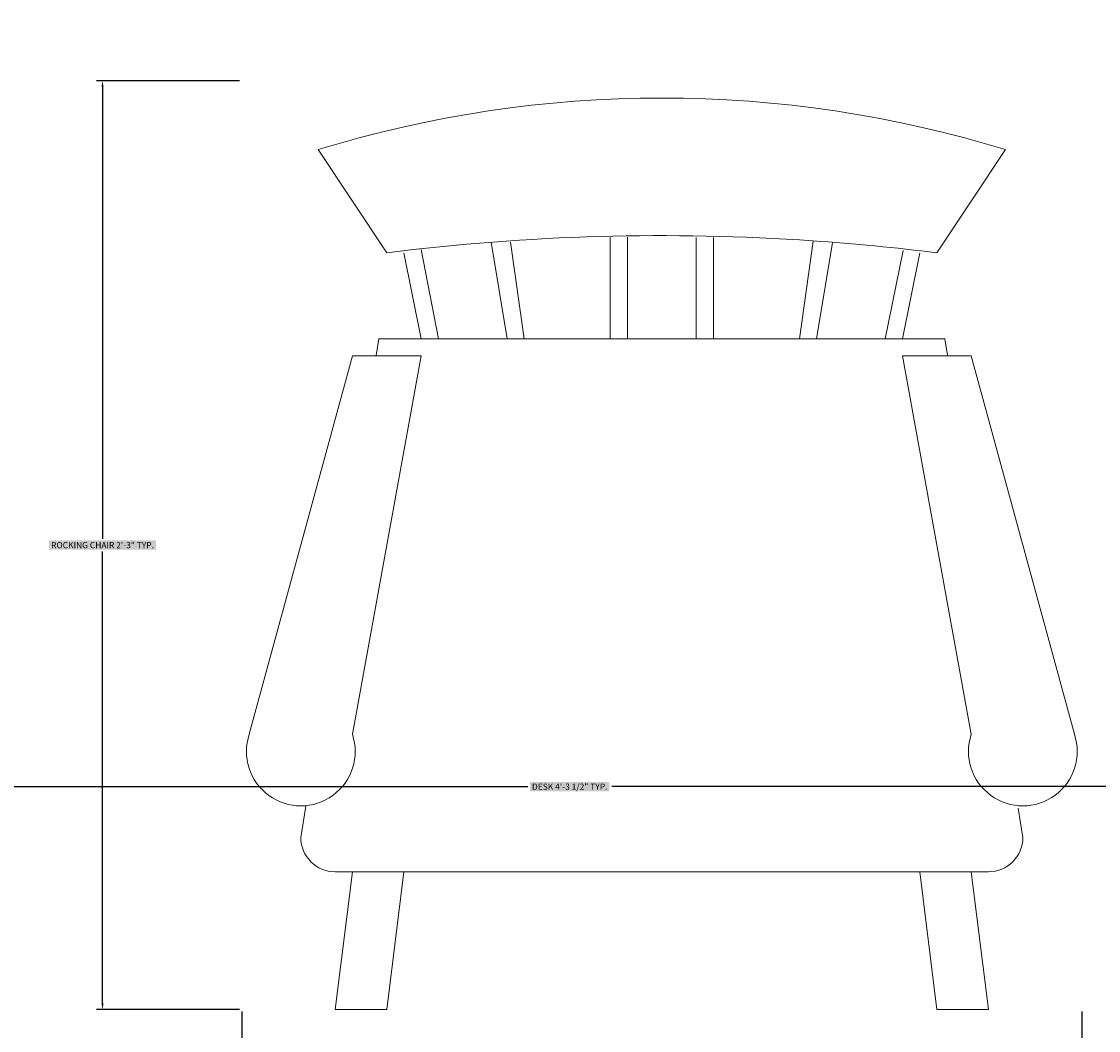
# Model space of a CAD drawing. Units: inches. Extents: x -301 to 715, y -607 to 364.
# Tile 81 of 141: x -94 to -62, y -39 to -10. Entities that reach past the tile are written whole.
import ezdxf

# ---------------------------------------------------------------- set-up
doc = ezdxf.new("R2010")
doc.units = ezdxf.units.IN
doc.header["$MEASUREMENT"] = 0
doc.layers.add('A-ANNO-DIMS', color=2, linetype='Continuous', lineweight=18)
doc.layers.add('A-FURN', color=8, linetype='Continuous', lineweight=18)
doc.styles.get("Standard").update_dxf_attribs({"font": 'arial.ttf'})
doc.dimstyles.get("Standard").update_dxf_attribs({"dimtxt": 0.18, "dimasz": 0.18, "dimexe": 0.18, "dimexo": 0.0625, "dimgap": 0.09, "dimtad": 0, "dimtih": 1, "dimtoh": 1, "dimdec": 1, "dimzin": 0, "dimdsep": 46, "dimlunit": 4, "dimtxsty": 'Standard', "dimcen": 0.09, "dimclrd": 3, "dimclre": 4, "dimclrt": 6, "dimadec": 0, "dimazin": 0, "dimtfac": 1, "dimtdec": 1, "dimtofl": 0, "dimtmove": 0, "dimatfit": 3, "dimfxl": 1, "dimtfill": 2, "dimtfillclr": 51, "dimtolj": 1, "dimtzin": 0, "dimarcsym": 0})

# ---------------------------------------------------------------- blocks, each defined once
blk = doc.blocks.new('Chair - Rocking')
for p, q in [((-8, -4.5), (-10, -1.5)), ((8, -4.5), (10, -1.5)), ((-1.5, -4.05012), (-1.5, -7)), ((-1, -7), (-1, -4.05012)), ((1, -7), (1, -4.04655)), ((1.5, -4.05012), (1.5, -7)), ((-4.5, -7), (-4.96674, -4.19951)), ((-4, -7), (-4.40532, -4.16272)), ((4, -7), (4.40187, -4.18694)), ((4.5, -7), (4.96761, -4.19437)), ((-7.5, -4.5), (-7, -7)), ((-6.5, -7), (-7.02225, -4.43)), ((6.5, -7), (7, -4.4057)), ((7.5, -4.5), (7, -7)), ((-8.23428, -6.99939), (-8.3093, -7.47958)), ((-8.23041, -7), (8.23915, -7)), ((8.31071, -7.48854), (8.23449, -7.00073)), ((-9, -7.5), (-12, -18.49999)), ((-7, -7.5), (-9, -7.5)), ((-9, -18.49999), (-7, -7.5)), ((7, -7.5), (9, -7.5)), ((9, -18.49999), (7, -7.5)), ((9, -7.5), (12, -18.49999)), ((-10.36644, -20.64523), (-10.5, -21.49999)), ((10.5, -21.49999), (10.3575, -20.58798)), ((-9, -22.49999), (-9.5, -26.49999)), ((0, -22.49999), (-9.5, -22.49999)), ((-8, -26.49999), (-7.5, -22.49999)), ((0, -22.49999), (9.5, -22.49999)), ((8, -26.49999), (7.5, -22.49999)), ((9, -22.49999), (9.5, -26.49999)), ((-9.5, -26.49999), (-8, -26.49999)), ((9.5, -26.49999), (8, -26.49999))]:
    blk.add_line(p, q)
for centre, radius, start, end in [((0, -34.08333), 34.08333, 72.93847, 107.0615), ((0, -68.25004), 64.25, 82.84733, 93.92211), ((0, -68.25004), 64.25, 93.92211, 97.15267), ((-10.5, -18.99999), 1.58114, 161.5651, 18.43495), ((10.5, -18.99999), 1.58114, 161.5651, 18.43495), ((-9.5, -21.49999), 1, 180, 270), ((9.5, -21.49999), 1, 270, 0)]:
    blk.add_arc(centre, radius, start, end)
blk = doc.blocks.new('*D114')
at = {"layer": 'A-ANNO-DIMS', "color": 4, "lineweight": -2, "transparency": 16777216}
for p, q in [((-103.477, -39.895), (-103.477, -32.076)), ((-52.128, -39.895), (-52.128, -32.076))]:
    blk.add_line(p, q, dxfattribs=at)
at = {"layer": 'A-ANNO-DIMS', "color": 3, "lineweight": -2, "transparency": 16777216}
for p, q in [((-103.297, -32.256), (-79.024, -32.256)), ((-52.308, -32.256), (-76.581, -32.256))]:
    blk.add_line(p, q, dxfattribs=at)
at = {"layer": 'A-ANNO-DIMS', "color": 3, "transparency": 16777216}
for points in [[(-103.297, -32.226), (-103.297, -32.286), (-103.477, -32.256)], [(-52.308, -32.226), (-52.308, -32.286), (-52.128, -32.256)]]:
    blk.add_solid(points, dxfattribs=at)
at = {"layer": 'Defpoints', "color": 0, "transparency": 16777216}
for p in [(-52.128, -32.256), (-103.477, -39.958), (-52.128, -39.958)]:
    blk.add_point(p, dxfattribs=at)
at = {"layer": 'A-ANNO-DIMS', "color": 6, "transparency": 16777216, "insert": (-77.803, -32.256), "char_height": 0.18, "attachment_point": 5, "bg_fill": 1, "box_fill_scale": 1.25, "bg_fill_color": 51, "bg_fill_transparency": 0}
blk.add_mtext('\\A1;DESK 4\'-3 1/2" TYP.', dxfattribs=at)
blk = doc.blocks.new('*D116')
at = {"layer": 'A-ANNO-DIMS', "color": 4, "lineweight": -2, "transparency": 16777216}
for p, q in [((-87.404, -11.733), (-91.571, -11.733)), ((-87.404, -38.733), (-91.571, -38.733))]:
    blk.add_line(p, q, dxfattribs=at)
at = {"layer": 'A-ANNO-DIMS', "color": 3, "lineweight": -2, "transparency": 16777216}
for p, q in [((-91.391, -11.913), (-91.391, -25.05)), ((-91.391, -38.553), (-91.391, -25.416))]:
    blk.add_line(p, q, dxfattribs=at)
at = {"layer": 'A-ANNO-DIMS', "color": 3, "transparency": 16777216}
for points in [[(-91.421, -11.913), (-91.361, -11.913), (-91.391, -11.733)], [(-91.421, -38.553), (-91.361, -38.553), (-91.391, -38.733)]]:
    blk.add_solid(points, dxfattribs=at)
at = {"layer": 'Defpoints', "color": 0, "transparency": 16777216}
for p in [(-91.391, -11.733), (-87.341, -11.733), (-87.341, -38.733)]:
    blk.add_point(p, dxfattribs=at)
at = {"layer": 'A-ANNO-DIMS', "color": 6, "transparency": 16777216, "insert": (-91.391, -25.233), "char_height": 0.18, "attachment_point": 5, "bg_fill": 1, "box_fill_scale": 1.25, "bg_fill_color": 51, "bg_fill_transparency": 0}
blk.add_mtext('\\A1;ROCKING CHAIR 2\'-3" TYP.', dxfattribs=at)
blk = doc.blocks.new('*D117')
at = {"layer": 'A-ANNO-DIMS', "color": 4, "lineweight": -2, "transparency": 16777216}
for p, q in [((-87.341, -38.796), (-87.341, -42.963)), ((-62.906, -38.796), (-62.906, -42.963))]:
    blk.add_line(p, q, dxfattribs=at)
at = {"layer": 'A-ANNO-DIMS', "color": 3, "lineweight": -2, "transparency": 16777216}
for p, q in [((-87.161, -42.783), (-75.974, -42.783)), ((-63.086, -42.783), (-74.274, -42.783))]:
    blk.add_line(p, q, dxfattribs=at)
at = {"layer": 'A-ANNO-DIMS', "color": 3, "transparency": 16777216}
for points in [[(-87.161, -42.753), (-87.161, -42.813), (-87.341, -42.783)], [(-63.086, -42.753), (-63.086, -42.813), (-62.906, -42.783)]]:
    blk.add_solid(points, dxfattribs=at)
at = {"layer": 'Defpoints', "color": 0, "transparency": 16777216}
for p in [(-87.341, -38.733), (-62.906, -38.733), (-87.341, -42.783)]:
    blk.add_point(p, dxfattribs=at)
at = {"layer": 'A-ANNO-DIMS', "color": 6, "transparency": 16777216, "insert": (-75.124, -42.783), "char_height": 0.18, "attachment_point": 5, "bg_fill": 1, "box_fill_scale": 1.25, "bg_fill_color": 51, "bg_fill_transparency": 0}
blk.add_mtext('\\A1;2\'-0 1/2" TYP.', dxfattribs=at)
blk = doc.blocks.new('*D151')
at = {"layer": 'A-ANNO-DIMS', "color": 4, "lineweight": -2, "transparency": 16777216}
for p, q in [((-204.603, -223.755), (-204.603, 359.612)), ((-45.603, -214.755), (-45.603, 359.612))]:
    blk.add_line(p, q, dxfattribs=at)
at = {"layer": 'A-ANNO-DIMS', "color": 3, "lineweight": -2, "transparency": 16777216}
for p, q in [((-204.423, 359.432), (-125.494, 359.432)), ((-45.783, 359.432), (-124.713, 359.432))]:
    blk.add_line(p, q, dxfattribs=at)
at = {"layer": 'A-ANNO-DIMS', "color": 3, "transparency": 16777216}
for points in [[(-204.423, 359.462), (-204.423, 359.402), (-204.603, 359.432)], [(-45.783, 359.462), (-45.783, 359.402), (-45.603, 359.432)]]:
    blk.add_solid(points, dxfattribs=at)
at = {"layer": 'Defpoints', "color": 0, "transparency": 16777216}
for p in [(-45.603, 359.432), (-45.603, -214.818), (-204.603, -223.818)]:
    blk.add_point(p, dxfattribs=at)
at = {"layer": 'A-ANNO-DIMS', "color": 6, "transparency": 16777216, "insert": (-125.103, 359.432), "char_height": 0.18, "attachment_point": 5, "bg_fill": 1, "box_fill_scale": 1.25, "bg_fill_color": 51, "bg_fill_transparency": 0}
blk.add_mtext('\\A1;13\'-3"', dxfattribs=at)
blk = doc.blocks.new('*D158')
at = {"layer": 'A-ANNO-DIMS', "color": 4, "lineweight": -2, "transparency": 16777216}
for p, q in [((-122.603, 221.62), (-122.603, -296.865)), ((-50.603, 221.62), (-50.603, -296.865))]:
    blk.add_line(p, q, dxfattribs=at)
at = {"layer": 'A-ANNO-DIMS', "color": 3, "lineweight": -2, "transparency": 16777216}
for p, q in [((-122.423, -296.685), (-86.933, -296.685)), ((-50.783, -296.685), (-86.274, -296.685))]:
    blk.add_line(p, q, dxfattribs=at)
at = {"layer": 'A-ANNO-DIMS', "color": 3, "transparency": 16777216}
for points in [[(-122.423, -296.655), (-122.423, -296.715), (-122.603, -296.685)], [(-50.783, -296.655), (-50.783, -296.715), (-50.603, -296.685)]]:
    blk.add_solid(points, dxfattribs=at)
at = {"layer": 'Defpoints', "color": 0, "transparency": 16777216}
for p in [(-122.603, 221.682), (-50.603, 221.682), (-50.603, -296.685)]:
    blk.add_point(p, dxfattribs=at)
at = {"layer": 'A-ANNO-DIMS', "color": 6, "transparency": 16777216, "insert": (-86.603, -296.685), "char_height": 0.18, "attachment_point": 5, "bg_fill": 1, "box_fill_scale": 1.25, "bg_fill_color": 51, "bg_fill_transparency": 0}
blk.add_mtext('\\A1;6\'-0"', dxfattribs=at)

msp = doc.modelspace()

# ---------------------------------------------------------------- block references
at = {"layer": 'A-FURN', "xscale": -1}
msp.add_blockref('Chair - Rocking', (-75.124, -12.233), dxfattribs=at)

# ---------------------------------------------------------------- dimensions: what is measured, and where the dimension line sits
at = {"layer": 'A-ANNO-DIMS'}
for base, p1, p2, picture, middle in [((-45.603, 359.432), (-204.603, -223.818), (-45.603, -214.818), '*D151', (-125.103, 359.432)), ((-50.603, -296.685), (-122.603, 221.682), (-50.603, 221.682), '*D158', (-86.603, -296.685))]:
    dim = msp.add_linear_dim(base=base, p1=p1, p2=p2, dimstyle='Standard', override={"dimdec": 1, "dimlfac": 1, "dimrnd": 0, "dimzin": 1, "dimdsep": 46, "dimlunit": 4, "dimfrac": 2}, dxfattribs=at)
    dim.commit()
    dim.dimension.update_dxf_attribs({"geometry": picture, "text_midpoint": middle})
for base, p1, p2, angle, text, picture, middle in [((-91.391, -11.733), (-87.341, -38.733), (-87.341, -11.733), 90, 'ROCKING CHAIR <> TYP.', '*D116', (-91.391, -25.233)), ((-87.341, -42.783), (-62.906, -38.733), (-87.341, -38.733), 180, '<> TYP.', '*D117', (-75.124, -42.783))]:
    dim = msp.add_linear_dim(base=base, p1=p1, p2=p2, angle=angle, text=text, dimstyle='Standard', override={"dimdec": 1, "dimlfac": 1, "dimrnd": 0, "dimzin": 1, "dimdsep": 46, "dimlunit": 4, "dimfrac": 2}, dxfattribs=at)
    dim.commit()
    dim.dimension.update_dxf_attribs({"geometry": picture, "text_midpoint": middle})
dim = msp.add_linear_dim(base=(-52.128, -32.256), p1=(-103.477, -39.958), p2=(-52.128, -39.958), text='DESK <> TYP.', dimstyle='Standard', override={"dimdec": 1, "dimlfac": 1, "dimrnd": 0, "dimzin": 1, "dimdsep": 46, "dimlunit": 4, "dimfrac": 2}, dxfattribs=at)
dim.commit()
dim.dimension.update_dxf_attribs({"geometry": '*D114', "text_midpoint": (-77.803, -32.256)})

doc.saveas('drawing.dxf')
